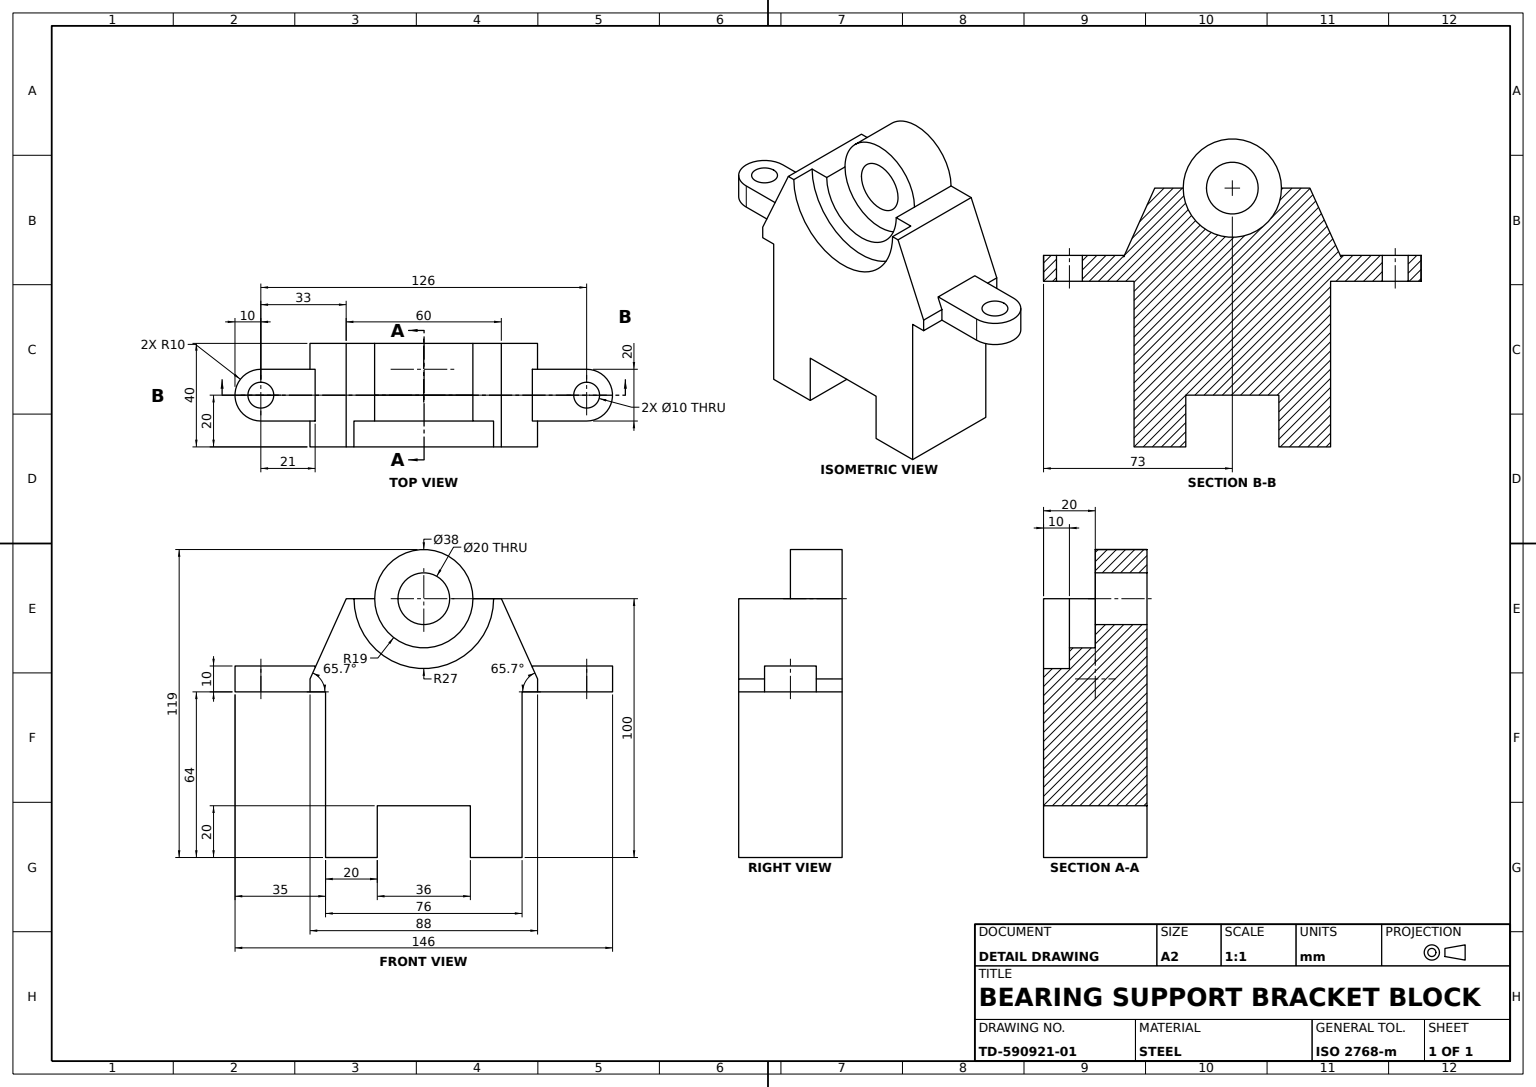
SolidWorks part; units mm, degrees
material "Plain Carbon Steel"
ref_plane "Front Plane" through (0, 0, 0) normal (0, 0, 1) x (1, 0, 0)
ref_plane "Top Plane" through (0, 0, 0) normal (0, 1, 0) x (1, 0, 0)
ref_plane "Right Plane" through (0, 0, 0) normal (1, 0, 0) x (0, 0, -1)
sketch "Base Body Sketch" plane through (0, 0, 0) normal (0, 0, 1) x (1, 0, 0)
  line L0 (0, 0) -> (0, 64)
  line L1 (0, 64) -> (76, 64)
  line L2 (76, 64) -> (76, 0)
  line L3 (76, 0) -> (56, 0)
  line L4 (56, 0) -> (56, 20)
  line L5 (56, 20) -> (20, 20)
  line L6 (20, 20) -> (20, 0)
  line L7 (20, 0) -> (0, 0)
  dimension "D1" = 20
  dimension "D2" = 56
  dimension "D3" = 64
extrude "Base Body" add sketch "Base Body Sketch" along normal blind 40
sketch "Upper Body Sketch" plane through (0, 0, 40) normal (0, 0, 1) x (1, 0, 0)
  line L0 (0, 64) -> (-6, 64)
  line L1 (-6, 64) -> (-6, 69)
  line L2 (56, 20) -> (56, 0) construction
  line L3 (20, 20) -> (56, 20) construction
  line L4 (38, 100) -> (68, 100)
  line L5 (38, 100) -> (8, 100)
  line L6 (8, 100) -> (-6, 69)
  line L7 (76, 64) -> (82, 64)
  line L8 (82, 64) -> (82, 69)
  line L9 (82, 69) -> (68, 100)
  line L10 (0, 64) -> (76, 64)
  dimension "D1" = 12
  dimension "D2" = 26
  dimension "D3" = 49
  dimension "D4" = 80
extrude "Upper Body" add sketch "Upper Body Sketch" against normal blind 40
sketch "Left Lug Block Sketch" plane through (-6, 0, 0) normal (-1, 0, 0) x (0, 0, 1)
  line L0 (40, 69) -> (40, 64) construction
  line L2 (0, 64) -> (40, 64) construction
  line L3 (30, 64) -> (30, 69)
  line L5 (30, 69) -> (10, 69)
  line L6 (0, 69) -> (40, 69) construction
  line L7 (10, 69) -> (10, 64)
  line L8 (10, 64) -> (30, 64)
  dimension "D1" = 10
  dimension "D2" = 30
extrude "Left Lug Block" add sketch "Left Lug Block Sketch" along normal blind 19
sketch "Left Lug Arm Sketch" plane through (-25, 0, 0) normal (-1, 0, 0) x (0, 0, 1)
  line L0 (10, 69) -> (10, 74)
  line L1 (10, 74) -> (30, 74)
  line L2 (30, 74) -> (30, 69)
  line L3 (30, 69) -> (10, 69) construction
  line L4 (30, 69) -> (10, 69)
  line L5 (10, 64) -> (30, 64) construction
  dimension "D1" = 10
extrude "Left Lug Arm" add sketch "Left Lug Arm Sketch" against normal blind 21
sketch "Left Lug End Sketch" plane through (0, 74, 0) normal (0, 1, 0) x (1, 0, 0)
  line L0 (-25, -30) -> (-25, -10) construction
  line L1 (-25, -10) -> (-25, -30)
  arc A0 (-25, -10) -> (-25, -30) centre (-25, -20) ccw
  dimension "D1" = 20
  dimension "D2" = 10
extrude "Left Lug Rounded End" add sketch "Left Lug End Sketch" against normal blind 10
sketch "Left Lug Hole Sketch" plane through (0, 74, 0) normal (0, 1, 0) x (1, 0, 0)
  circle A0 centre (-25, -20) radius 5
  dimension "D1" = 10
  dimension "D2" = 10
extrude "Left Lug Hole Ø10" cut sketch "Left Lug Hole Sketch" against normal blind 10
sketch "Right Lug Block Sketch" plane through (82, 0, 0) normal (1, 0, 0) x (0, 0, -1)
  line L0 (-40, 64) -> (-40, 69) construction
  line L1 (0, 64) -> (-40, 64) construction
  line L2 (-10, 64) -> (-10, 69)
  line L4 (-10, 69) -> (-30, 69)
  line L5 (0, 69) -> (-40, 69) construction
  line L6 (-30, 69) -> (-30, 64)
  line L7 (-30, 64) -> (-10, 64)
  dimension "D1" = 10
  dimension "D2" = 30
extrude "Right Lug Block" add sketch "Right Lug Block Sketch" along normal blind 19
sketch "Right Lug Arm Sketch" plane through (101, 0, 0) normal (1, 0, 0) x (0, 0, -1)
  line L0 (-30, 69) -> (-30, 74)
  line L1 (-30, 74) -> (-10, 74)
  line L2 (-10, 74) -> (-10, 69)
  line L3 (-10, 69) -> (-30, 69)
  line L4 (-30, 64) -> (-10, 64) construction
  dimension "D1" = 10
extrude "Right Lug Arm" add sketch "Right Lug Arm Sketch" against normal blind 21
sketch "Right Lug End Sketch" plane through (0, 74, 0) normal (0, 1, 0) x (1, 0, 0)
  line L0 (101, -10) -> (101, -30) construction
  line L1 (101, -10) -> (101, -30)
  arc A0 (101, -30) -> (101, -10) centre (101, -20) ccw
  dimension "D1" = 20
extrude "Right Lug Rounded End" add sketch "Right Lug End Sketch" against normal blind 10
sketch "Right Lug Hole Sketch" plane through (0, 74, 0) normal (0, 1, 0) x (1, 0, 0)
  circle A0 centre (101, -20) radius 5
  dimension "D1" = 10
  dimension "D2" = 10
extrude "Right Lug Hole Ø10" cut sketch "Right Lug Hole Sketch" against normal blind 10
sketch "Bearing Seat Sketch" plane through (0, 0, 40) normal (0, 0, 1) x (1, 0, 0)
  line L0 (68, 100) -> (8, 100) construction
  line L1 (11, 100) -> (65, 100)
  arc A0 (11, 100) -> (65, 100) centre (38, 100) ccw
  dimension "D1" = 54
  dimension "D2" = 27
extrude "Bearing Seat Cut Ø54" cut sketch "Bearing Seat Sketch" against normal blind 10
sketch "Seat Groove Sketch" plane through (0, 0, 30) normal (0, 0, 1) x (1, 0, 0)
  line L0 (19, 100) -> (57, 100)
  arc A0 (19, 100) -> (57, 100) centre (38, 100) ccw
  dimension "D1" = 38
  dimension "D2" = 19
extrude "Seat Groove Ø38" cut sketch "Seat Groove Sketch" against normal blind 30
sketch "Hub Sketch" plane through (0, 0, 30) normal (0, 0, 1) x (1, 0, 0)
  circle A0 centre (38, 100) radius 19
  dimension "D1" = 38
  dimension "D2" = 38
  dimension "D3" = 38
  dimension "D4" = 100
extrude "Hub Ø38" add sketch "Hub Sketch" against normal blind 30
sketch "Hub Recess Sketch" plane through (0, 0, 30) normal (0, 0, 1) x (1, 0, 0)
  circle A0 centre (38, 100) radius 19
  dimension "D1" = 38
  dimension "D2" = 38
extrude "Hub Recess Ø38" cut sketch "Hub Recess Sketch" against normal blind 10
sketch "Bore Sketch" plane through (0, 0, 20) normal (0, 0, 1) x (1, 0, 0)
  circle A0 centre (38, 100) radius 10
  dimension "D1" = 20
  dimension "D2" = 20
extrude "Bore Ø20" cut sketch "Bore Sketch" against normal blind 20
